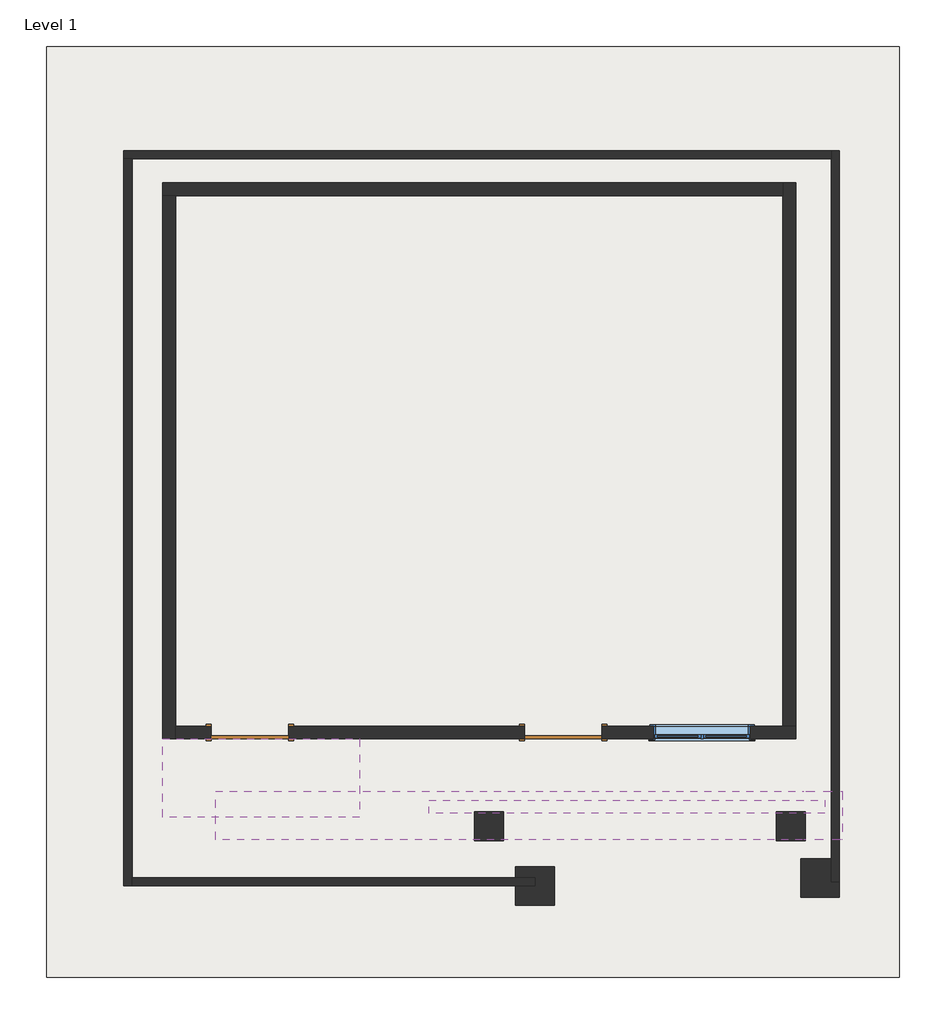
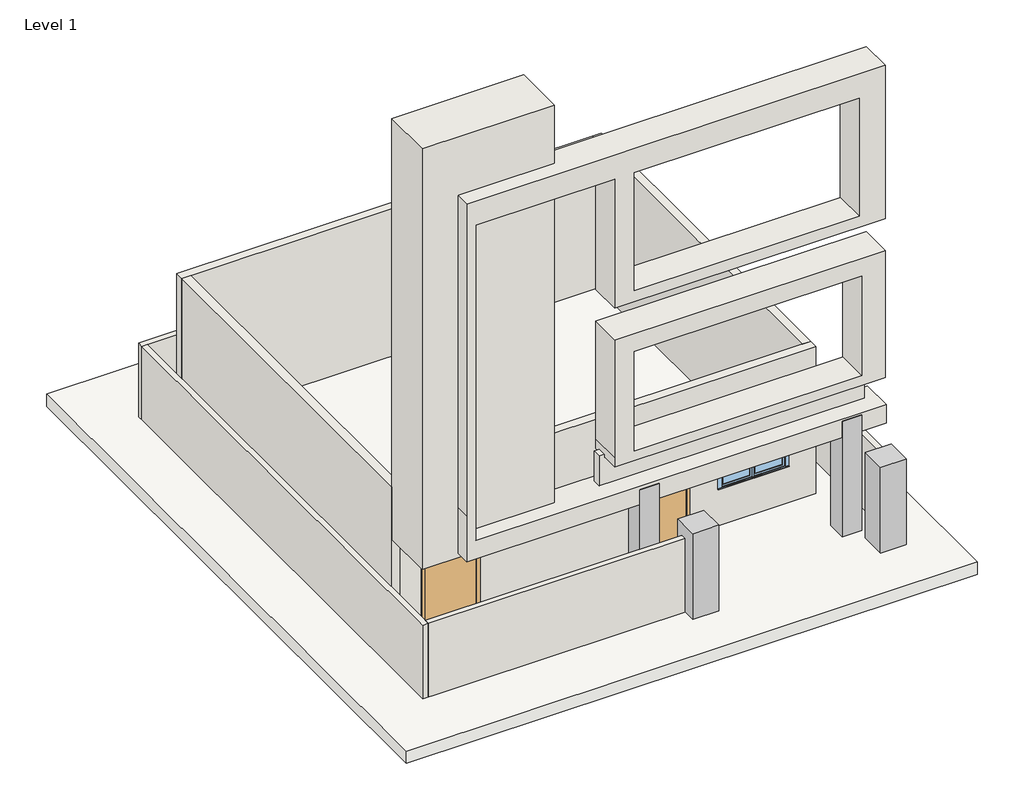
# One storey: 11 walls, 4 columns, 2 doors, 1 slab, 1 window.
"""IFC4 building model written with IfcOpenShell, lengths in millimetres."""

from ifc_helpers import new_model, si_unit, frame, origin, origin_with_axes, place, context, project, spatial, polyline, outline, extrude, faceted_brep, transform, mapped, element, save
from components import door_ba16a7d3, walls_1_walls_1_cc25df17, walls_2_walls_2_595a3e20, window_03976a38

model = new_model("IFC4")

# Units and contexts
model_context = context("Model", 3, world=origin())
ifc_project = project(units=[si_unit("LENGTHUNIT", "METRE", prefix="MILLI")], contexts=[model_context])

# Site, building, storey
site = spatial("IfcSite", under=ifc_project)
building = spatial("IfcBuilding", under=site)
storey = spatial("IfcBuildingStorey", under=building, Name="Level 1", Elevation=0.0)

# Columns
placement = place(None, origin())
element("IfcColumn", 1, ObjectType="Rectangular Column : 18\" x 18\"", at=placement, inside=storey, context=model_context, shape_type="SweptSolid", body=[
    extrude(outline(polyline([(-3346.1936733, 3595.4419215), (-3346.1936733, 3138.2419215), (-3803.3936733, 3138.2419215), (-3803.3936733, 3595.4419215), (-3346.1936733, 3595.4419215)])), origin_with_axes(), (0.0, 0.0, 1.0), 2834.6796875),
])
element("IfcColumn", 2, ObjectType="Rectangular Column : 18\" x 18\"", at=placement, inside=storey, context=model_context, shape_type="SweptSolid", body=[
    extrude(outline(polyline([(1403.6063267, 3595.4419215), (1403.6063267, 3138.2419215), (946.4063267, 3138.2419215), (946.4063267, 3595.4419215), (1403.6063267, 3595.4419215)])), origin_with_axes(), (0.0, 0.0, 1.0), 2870.2),
])
element("IfcColumn", 3, ObjectType="Rectangular Column : 24\" x 24\"", at=placement, inside=storey, context=model_context, shape_type="Brep", body=[
    faceted_brep([(-2544.2183312, 2732.2634766, 2133.6), (-3153.8183312, 2732.2634766, 2133.6), (-3153.8183312, 2122.6634766, 2133.6), (-2544.2183312, 2122.6634766, 2133.6), (-2544.2183312, 2732.2634766, 0.0), (-2544.2183312, 2122.6634766, 0.0), (-3153.8183312, 2122.6634766, 0.0), (-3153.8183312, 2427.4634766, 0.0), (-2849.0183312, 2427.4634766, 0.0), (-2849.0183312, 2554.4634766, 0.0), (-3153.8183312, 2554.4634766, 0.0), (-3153.8183312, 2732.2634766, 0.0), (-3153.8183312, 2554.4634766, 1828.8), (-3153.8183312, 2427.4634766, 1828.8), (-2849.0183312, 2554.4634766, 1828.8), (-2849.0183312, 2427.4634766, 1828.8)], [[[0, 1, 2, 3]], [[4, 5, 6, 7, 8, 9, 10, 11]], [[1, 0, 4, 11]], [[2, 1, 11, 10, 12, 13, 7, 6]], [[3, 2, 6, 5]], [[0, 3, 5, 4]], [[9, 14, 12, 10]], [[15, 8, 7, 13]], [[14, 15, 13, 12]], [[14, 9, 8, 15]]]),
])
element("IfcColumn", 4, ObjectType="Rectangular Column : 24\" x 24\"", at=placement, inside=storey, context=model_context, shape_type="Brep", body=[
    faceted_brep([(1938.8816688, 2858.8419215, 2133.6), (1329.2816688, 2858.8419215, 2133.6), (1329.2816688, 2249.2419215, 2133.6), (1938.8816688, 2249.2419215, 2133.6), (1938.8816688, 2249.2419215, 0.0), (1329.2816688, 2249.2419215, 0.0), (1329.2816688, 2858.8419215, 0.0), (1811.8816688, 2858.8419215, 0.0), (1811.8816688, 2490.9634766, 0.0), (1938.8816688, 2490.9634766, 0.0), (1938.8816688, 2858.8419215, 1828.8), (1811.8816688, 2858.8419215, 1828.8), (1938.8816688, 2490.9634766, 1828.8), (1811.8816688, 2490.9634766, 1828.8)], [[[0, 1, 2, 3]], [[4, 5, 6, 7, 8, 9]], [[1, 0, 10, 11, 7, 6]], [[2, 1, 6, 5]], [[3, 2, 5, 4]], [[0, 3, 4, 9, 12, 10]], [[13, 8, 7, 11]], [[8, 13, 12, 9]], [[12, 13, 11, 10]]]),
])

# Doors
door_shape = door_ba16a7d3(model_context)
element("IfcDoor", 5, ObjectType="Single-Flush : 36\" x 84\"", at=placement, inside=storey, context=model_context, shape_type="MappedRepresentation", body=[
    mapped(door_shape, transform((-2406.3936733, 4840.0419215, 0.0), x_axis=(-1.0, 0.0, 0.0), y_axis=(0.0, -1.0, 0.0), z_axis=(0.0, 0.0, 1.0))),
])
element("IfcDoor", 6, ObjectType="Single-Flush : 36\" x 84\"", at=placement, inside=storey, context=model_context, shape_type="MappedRepresentation", body=[
    mapped(door_shape, transform((-7333.9936733, 4840.0419215, 0.0), x_axis=(-1.0, 0.0, 0.0), y_axis=(0.0, -1.0, 0.0), z_axis=(0.0, 0.0, 1.0))),
])

# Slab
element("IfcSlab", 7, ObjectType="Generic - 12\"", at=placement, inside=storey, context=model_context, shape_type="SweptSolid", body=[
    extrude(outline(polyline([(2881.7690782, 15620.785378), (2881.7690782, 990.385378), (-10529.4309218, 990.385378), (-10529.4309218, 15620.785378), (2881.7690782, 15620.785378)])), frame((0.0, 0.0, -304.8), z_axis=(0.0, 0.0, 1.0), x_axis=(1.0, 0.0, 0.0)), (0.0, 0.0, 1.0), 304.8),
])

# Walls
element("IfcWall", 8, ObjectType="Generic - 5\"", at=placement, inside=storey, context=model_context, shape_type="Brep", body=[
    faceted_brep([(-9313.3183312, 13857.4634766, 0.0), (-9186.3183312, 13857.4634766, 0.0), (1811.8816688, 13857.4634766, 0.0), (1811.8816688, 13857.4634766, 1828.8), (-9186.3183312, 13857.4634766, 1828.8), (-9313.3183312, 13857.4634766, 1828.8), (-9313.3183312, 13984.4634766, 0.0), (-9313.3183312, 13984.4634766, 1828.8), (1811.8816688, 13984.4634766, 1828.8), (1811.8816688, 13984.4634766, 0.0)], [[[0, 1, 2, 3, 4, 5]], [[6, 7, 8, 9]], [[2, 1, 0, 6, 9]], [[5, 4, 3, 8, 7]], [[0, 5, 7, 6]], [[3, 2, 9, 8]]]),
])
element("IfcWall", 9, ObjectType="Generic - 5\"", at=placement, inside=storey, context=model_context, shape_type="Brep", body=[
    faceted_brep([(-9186.3183312, 2427.4634766, 0.0), (-9186.3183312, 2554.4634766, 0.0), (-9186.3183312, 13857.4634766, 0.0), (-9186.3183312, 13857.4634766, 1828.8), (-9186.3183312, 2554.4634766, 1828.8), (-9186.3183312, 2427.4634766, 1828.8), (-9313.3183312, 2427.4634766, 0.0), (-9313.3183312, 2427.4634766, 1828.8), (-9313.3183312, 13857.4634766, 1828.8), (-9313.3183312, 13857.4634766, 0.0)], [[[0, 1, 2, 3, 4, 5]], [[6, 7, 8, 9]], [[2, 1, 0, 6, 9]], [[5, 4, 3, 8, 7]], [[0, 5, 7, 6]], [[3, 2, 9, 8]]]),
])
element("IfcWall", 10, ObjectType="Generic - 5\"", at=placement, inside=storey, context=model_context, shape_type="Brep", body=[
    faceted_brep([(-2849.0183312, 2554.4634766, 0.0), (-3153.8183312, 2554.4634766, 0.0), (-9186.3183312, 2554.4634766, 0.0), (-9186.3183312, 2554.4634766, 1828.8), (-3153.8183312, 2554.4634766, 1828.8), (-2849.0183312, 2554.4634766, 1828.8), (-2849.0183312, 2427.4634766, 0.0), (-2849.0183312, 2427.4634766, 1828.8), (-3153.8183312, 2427.4634766, 1828.8), (-9186.3183312, 2427.4634766, 1828.8), (-9186.3183312, 2427.4634766, 0.0), (-3153.8183312, 2427.4634766, 0.0)], [[[0, 1, 2, 3, 4, 5]], [[6, 7, 8, 9, 10, 11]], [[2, 1, 0, 6, 11, 10]], [[5, 4, 3, 9, 8, 7]], [[0, 5, 7, 6]], [[3, 2, 10, 9]]]),
])
element("IfcWall", 11, ObjectType="Generic - 5\"", at=placement, inside=storey, context=model_context, shape_type="Brep", body=[
    faceted_brep([(1811.8816688, 13984.4634766, 0.0), (1811.8816688, 13857.4634766, 0.0), (1811.8816688, 2858.8419215, 0.0), (1811.8816688, 2490.9634766, 0.0), (1811.8816688, 2490.9634766, 1828.8), (1811.8816688, 2858.8419215, 1828.8), (1811.8816688, 13857.4634766, 1828.8), (1811.8816688, 13984.4634766, 1828.8), (1938.8816688, 13984.4634766, 0.0), (1938.8816688, 13984.4634766, 1828.8), (1938.8816688, 2858.8419215, 1828.8), (1938.8816688, 2490.9634766, 1828.8), (1938.8816688, 2490.9634766, 0.0)], [[[0, 1, 2, 3, 4, 5, 6, 7]], [[8, 9, 10, 11, 12]], [[3, 2, 1, 0, 8, 12]], [[4, 3, 12, 11]], [[7, 6, 5, 4, 11, 10, 9]], [[0, 7, 9, 8]]]),
])
element("IfcWall", 12, ObjectType="Generic - 8\"", at=placement, inside=storey, context=model_context, shape_type="Brep", body=[
    faceted_brep([(-8705.5936733, 13272.8419215, 0.0), (-8502.3936733, 13272.8419215, 0.0), (1048.0063267, 13272.8419215, 0.0), (1048.0063267, 13272.8419215, 3657.6), (-8502.3936733, 13272.8419215, 3657.6), (-8705.5936733, 13272.8419215, 3657.6), (-8705.5936733, 13476.0419215, 0.0), (-8705.5936733, 13476.0419215, 3657.6), (1048.0063267, 13476.0419215, 3657.6), (1048.0063267, 13476.0419215, 0.0)], [[[0, 1, 2, 3, 4, 5]], [[6, 7, 8, 9]], [[2, 1, 0, 6, 9]], [[0, 5, 7, 6]], [[3, 2, 9, 8]], [[5, 4, 3, 8, 7]]]),
])
element("IfcWall", 13, ObjectType="Generic - 8\"", at=placement, inside=storey, context=model_context, shape_type="Brep", body=[
    faceted_brep([(-8502.3936733, 4738.4419215, 0.0), (-8502.3936733, 4941.6419215, 0.0), (-8502.3936733, 13272.8419215, 0.0), (-8502.3936733, 13272.8419215, 3657.6), (-8502.3936733, 4941.6419215, 3657.6), (-8502.3936733, 4738.4419215, 3657.6), (-8705.5936733, 4738.4419215, 0.0), (-8705.5936733, 4738.4419215, 3657.6), (-8705.5936733, 13272.8419215, 3657.6), (-8705.5936733, 13272.8419215, 0.0)], [[[0, 1, 2, 3, 4, 5]], [[6, 7, 8, 9]], [[2, 1, 0, 6, 9]], [[0, 5, 7, 6]], [[3, 2, 9, 8]], [[5, 4, 3, 8, 7]]]),
])
element("IfcWall", 14, ObjectType="Generic - 8\"", at=placement, inside=storey, context=model_context, shape_type="Brep", body=[
    faceted_brep([(-7943.5936733, 4941.6419215, 2133.6), (-7943.5936733, 4941.6419215, 0.0), (-8502.3936733, 4941.6419215, 0.0), (-8502.3936733, 4941.6419215, 3657.6), (1048.0063267, 4941.6419215, 3657.6), (1251.2063267, 4941.6419215, 3657.6), (1251.2063267, 4941.6419215, 0.0), (1048.0063267, 4941.6419215, 0.0), (-1796.7936733, 4941.6419215, 0.0), (-1796.7936733, 4941.6419215, 2133.6), (-3015.9936733, 4941.6419215, 2133.6), (-3015.9936733, 4941.6419215, 0.0), (-6724.3936733, 4941.6419215, 0.0), (-6724.3936733, 4941.6419215, 2133.6), (-983.9936733, 4941.6419215, 2133.6), (-983.9936733, 4941.6419215, 914.4), (540.0063267, 4941.6419215, 914.4), (540.0063267, 4941.6419215, 2133.6), (-8502.3936733, 4738.4419215, 0.0), (-7943.5936733, 4738.4419215, 0.0), (-7943.5936733, 4738.4419215, 2133.6), (-6724.3936733, 4738.4419215, 2133.6), (-6724.3936733, 4738.4419215, 0.0), (-3015.9936733, 4738.4419215, 0.0), (-3015.9936733, 4738.4419215, 2133.6), (-1796.7936733, 4738.4419215, 2133.6), (-1796.7936733, 4738.4419215, 0.0), (1251.2063267, 4738.4419215, 0.0), (1251.2063267, 4738.4419215, 3657.6), (-8502.3936733, 4738.4419215, 3657.6), (-983.9936733, 4738.4419215, 2133.6), (540.0063267, 4738.4419215, 2133.6), (540.0063267, 4738.4419215, 914.4), (-983.9936733, 4738.4419215, 914.4)], [[[0, 1, 2, 3, 4, 5, 6, 7, 8, 9, 10, 11, 12, 13], [14, 15, 16, 17]], [[18, 19, 20, 21, 22, 23, 24, 25, 26, 27, 28, 29], [30, 31, 32, 33]], [[8, 7, 6, 27, 26]], [[12, 11, 23, 22]], [[2, 1, 19, 18]], [[6, 5, 28, 27]], [[3, 2, 18, 29]], [[5, 4, 3, 29, 28]], [[24, 23, 11, 10]], [[25, 24, 10, 9]], [[26, 25, 9, 8]], [[15, 14, 30, 33]], [[16, 15, 33, 32]], [[17, 16, 32, 31]], [[14, 17, 31, 30]], [[20, 19, 1, 0]], [[21, 20, 0, 13]], [[22, 21, 13, 12]]]),
])
element("IfcWall", 15, ObjectType="Generic - 8\"", at=placement, inside=storey, context=model_context, shape_type="Brep", body=[
    faceted_brep([(1048.0063267, 13476.0419215, 0.0), (1048.0063267, 13272.8419215, 0.0), (1048.0063267, 4941.6419215, 0.0), (1048.0063267, 4941.6419215, 3657.6), (1048.0063267, 13272.8419215, 3657.6), (1048.0063267, 13476.0419215, 3657.6), (1251.2063267, 13476.0419215, 0.0), (1251.2063267, 13476.0419215, 3657.6), (1251.2063267, 4941.6419215, 3657.6), (1251.2063267, 4941.6419215, 0.0)], [[[0, 1, 2, 3, 4, 5]], [[6, 7, 8, 9]], [[2, 1, 0, 6, 9]], [[0, 5, 7, 6]], [[3, 2, 9, 8]], [[5, 4, 3, 8, 7]]]),
])
element("IfcWall", 16, ObjectType="Generic - 8\"", at=placement, inside=storey, context=model_context, shape_type="SweptSolid", body=[
    extrude(outline(polyline([(1708.4063267, 3570.0419215), (-4514.5936733, 3570.0419215), (-4514.5936733, 3773.2419215), (1708.4063267, 3773.2419215), (1708.4063267, 3570.0419215)])), frame((0.0, 0.0, 2921.0), z_axis=(0.0, 0.0, 1.0), x_axis=(1.0, 0.0, 0.0)), (0.0, 0.0, 1.0), 736.6),
])
walls_1_walls_1_shape = walls_1_walls_1_cc25df17(model_context)
element("IfcWall", 17, ObjectType="Walls 1 : Walls 1", at=placement, inside=storey, context=model_context, shape_type="MappedRepresentation", body=[
    mapped(walls_1_walls_1_shape, transform((0.0, 0.0, 0.0), x_axis=(1.0, 0.0, 0.0), y_axis=(0.0, 1.0, 0.0), z_axis=(0.0, 0.0, 1.0))),
])
walls_2_walls_2_shape = walls_2_walls_2_595a3e20(model_context)
element("IfcWall", 18, ObjectType="Walls 2 : Walls 2", at=placement, inside=storey, context=model_context, shape_type="MappedRepresentation", body=[
    mapped(walls_2_walls_2_shape, transform((0.0, 0.0, 0.0), x_axis=(1.0, 0.0, 0.0), y_axis=(0.0, 1.0, 0.0), z_axis=(0.0, 0.0, 1.0))),
])

# Window
window_shape = window_03976a38(model_context)
element("IfcWindow", 19, ObjectType="Casement Dbl with Trim : 48\" x 48\"", at=placement, inside=storey, context=model_context, shape_type="MappedRepresentation", body=[
    mapped(window_shape, transform((-221.9936733, 4859.0919215, 0.0), x_axis=(-1.0, 0.0, 0.0), y_axis=(0.0, -1.0, 0.0), z_axis=(0.0, 0.0, 1.0))),
])

save(model, "model.ifc")

# Revit data of these elements
# Type "Rectangular Column : 18\" x 18\""
#   Assembly Code = "B1010200"
#   Depth = 1' - 6"
#   Offset Base = 0' - 0"
#   Offset Top = 0' - 0"
#   Width = 1' - 6"
#   Material = none
# Type "Rectangular Column : 24\" x 24\""
#   Assembly Code = "B1010200"
#   Depth = 2' - 0"
#   Offset Base = 0' - 0"
#   Offset Top = 0' - 0"
#   Width = 2' - 0"
#   Material = none
# Type "Single-Flush : 36\" x 84\""
#   Type Mark = "1"
#   Construction Type Id = "MDOOR"
#   Assembly Code = "C1020"
#   Analytic Construction = "Metal"
#   Thickness = 0' - 2"
#   Heat Transfer Coefficient (U) = 0.651978 BTU/(h·ft²·°F)
#   Height = 7' - 0"
#   Trim Projection Ext = 0' - 1"
#   Trim Projection Int = 0' - 1"
#   Trim Width = 0' - 3"
#   Width = 4' - 0"
#   Define Thermal Properties by = 1
#   Door Material = Door - Panel
#   Frame Material = Door - Frame
#   Visual Light Transmittance = 0
#   Solar Heat Gain Coefficient = 0
#   Function = (empty or 0)
#   Wall Closure = (empty or 0)
# Type "Generic - 12\""
#   Assembly Code = "B1010"
#   Function = 0
#   Layers, outside or top first: 1' - 0" no material (function 1)
# Type "Generic - 5\""
#   Assembly Code = "B2010"
#   Layers, outside or top first: 0' - 5" no material (function 1)
# Type "Generic - 8\""
#   Assembly Code = "B2010"
#   Layers, outside or top first: 0' - 8" no material (function 1)
# Type "Casement Dbl with Trim : 48\" x 48\""
#   Type Mark = "10"
#   Construction Type Id = "GSP4R"
#   Assembly Code = "B2020100"
#   Analytic Construction = "1/8 in Pilkington single glazing"
#   Visual Light Transmittance = 0.9
#   Solar Heat Gain Coefficient = 0.78
#   Heat Transfer Coefficient (U) = 0.6496 BTU/(h·ft²·°F)
#   Height = 4' - 0"
#   Default Sill Height = 3' - 0"
#   Trim Projection - Ext. = 0' - 0 1/2"
#   Trim Projection - Int. = 0' - 0 3/4"
#   Trim Width - Exterior = 0' - 3 1/2"
#   Trim Width - Interior = 0' - 3 1/2"
#   Width = 5' - 0"
#   Window Inset = 0' - 0 3/4"
#   Define Thermal Properties by = 1
#   Glass Pane Material = Glass
#   Sash Material = Sash
#   Trim Exterior Material = Trim
#   Trim Interior Material = Trim
#   Wall Closure = (empty or 0)
# Elements 1, 2 (IfcColumn, "Rectangular Column : 18\" x 18\"")
#   Phase Created = New Construction
# Elements 3, 4 (IfcColumn, "Rectangular Column : 24\" x 24\"")
#   Phase Created = New Construction
#   Materials on its faces: "Default Wall"
# Elements 5, 6 (IfcDoor, "Single-Flush : 36\" x 84\"")
#   Phase Created = New Construction
#   Materials on its faces: "Door - Frame", "Door - Panel"
# Element 7 (IfcSlab, "Generic - 12\"")
#   Height Offset From Level = 0' - 0"
#   Phase Created = New Construction
#   Materials on its faces: "Default Floor"
# Elements 8, 9, 10, 11 (IfcWall, "Generic - 5\"")
#   Top Offset = -6' - 0"
#   Base Offset = 0' - 0"
#   wall height = 6' - 0"
#   Phase Created = New Construction
#   Base Constraint = Level 1
#   Top Constraint = Level 2
#   Materials on its faces: "Default Wall"
# Elements 12, 13, 14, 15 (IfcWall, "Generic - 8\"")
#   Top Offset = 0' - 0"
#   Base Offset = 0' - 0"
#   Unconnected Height = 12' - 0"
#   wall height = 12' - 0"
#   Phase Created = New Construction
#   Base Constraint = Level 1
#   Materials on its faces: "Default Wall"
# Element 16 (IfcWall, "Generic - 8\"")
#   built-in parameter 1001111 = 9' - 7"
#   Top Offset = 0' - 0"
#   Base Offset = 9' - 7"
#   Unconnected Height = 2' - 5"
#   wall height = 2' - 5"
#   Phase Created = New Construction
#   Base Constraint = Level 1
#   Materials on its faces: "Default Wall"
# Element 17 (IfcWall, "Walls 1 : Walls 1")
#   Phase Created = New Construction
#   Materials on its faces: "Default Wall"
# Element 18 (IfcWall, "Walls 2 : Walls 2")
#   Phase Created = New Construction
#   Materials on its faces: "Default Wall"
# Element 19 (IfcWindow, "Casement Dbl with Trim : 48\" x 48\"")
#   Mark = "2"
#   Phase Created = New Construction
#   Materials on its faces: "Sash", "Trim", "Glass"
# Materials
#   "Door - Panel": class "Wood", colour RGB 210 159 95, transparency 0
#   "Door - Frame": colour RGB 118 70 51, transparency 0
#   "Glass": class "Glass", colour RGB 0 128 192, transparency 0.75, Description = "Soda Lime Glass", Cost = 0
#   "Sash": class "Wood", colour RGB 224 178 126, transparency 0
#   "Trim": class "Wood", colour RGB 224 178 126, transparency 0
#   "Default Wall": colour RGB 128 128 128, transparency 0
#   "Default Floor": colour RGB 128 128 128, transparency 0
